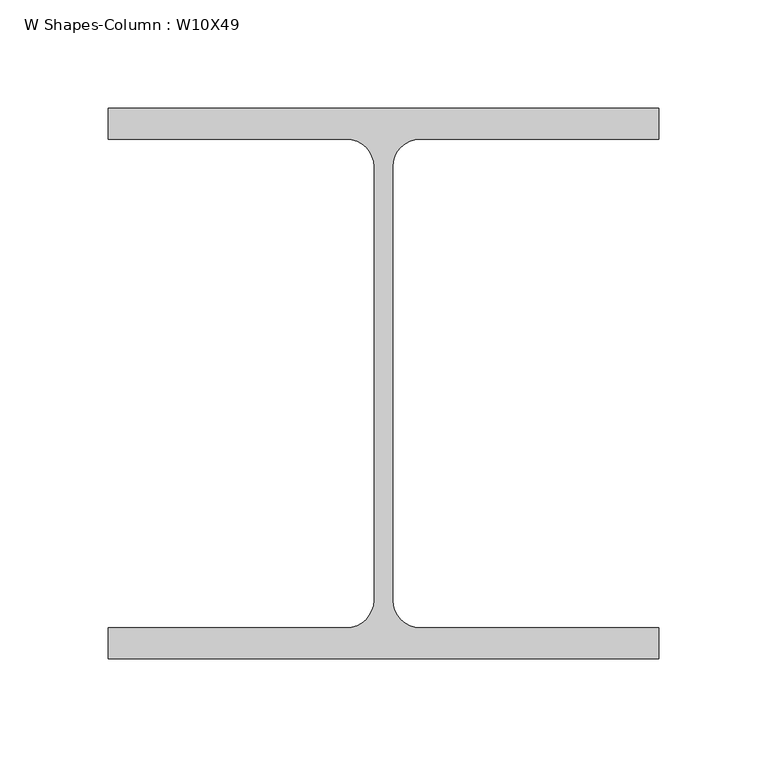
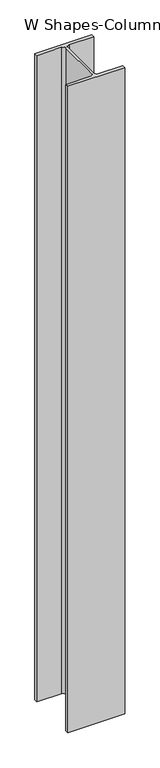
"""IFC4 building model written with IfcOpenShell, lengths in millimetres: column geometry, W Shapes-Column : W10X49."""

from ifc_helpers import new_model, si_unit, point, frame_2d, origin, origin_with_axes, place, context, project, spatial, polyline, circle_curve, trimmed, segment, composite_curve, outline, extrude, source, transform, mapped, element, save


def w_shapes_column_w10x49_a631470e(model_context):
    return source(origin(), model_context, "Body", "SweptSolid", [
        extrude(outline(composite_curve([segment(polyline([(127.0, 127.0), (127.0, 112.776), (17.018, 112.776)]), True, "CONTINUOUS"), segment(trimmed(circle_curve(frame_2d((17.018, 100.076)), 12.7), [point((17.018, 112.776))], [point((4.318, 100.076))], True, "CARTESIAN"), True, "CONTINUOUS"), segment(polyline([(4.318, 100.076), (4.318, -100.076)]), True, "CONTINUOUS"), segment(trimmed(circle_curve(frame_2d((17.018, -100.076)), 12.7), [point((4.318, -100.076))], [point((17.018, -112.776))], True, "CARTESIAN"), True, "CONTINUOUS"), segment(polyline([(17.018, -112.776), (127.0, -112.776), (127.0, -127.0), (-127.0, -127.0), (-127.0, -112.776), (-17.018, -112.776)]), True, "CONTINUOUS"), segment(trimmed(circle_curve(frame_2d((-17.018, -100.076)), 12.7), [point((-17.018, -112.776))], [point((-4.318, -100.076))], True, "CARTESIAN"), True, "CONTINUOUS"), segment(polyline([(-4.318, -100.076), (-4.318, 100.076)]), True, "CONTINUOUS"), segment(trimmed(circle_curve(frame_2d((-17.018, 100.076)), 12.7), [point((-4.318, 100.076))], [point((-17.018, 112.776))], True, "CARTESIAN"), True, "CONTINUOUS"), segment(polyline([(-17.018, 112.776), (-127.0, 112.776), (-127.0, 127.0), (127.0, 127.0)]), True, "CONTINUOUS")], self_intersect=False)), origin_with_axes(), (0.0, 0.0, 1.0), 3048.0),
    ])


if __name__ == "__main__":
    model = new_model("IFC4")
    model_context = context("Model", 3, world=origin())
    ifc_project = project(units=[si_unit("LENGTHUNIT", "METRE", prefix="MILLI")], contexts=[model_context])
    site = spatial("IfcSite", under=ifc_project)
    building = spatial("IfcBuilding", under=site)
    placement = place(None, origin())
    w_shapes_column_w10x49_shape = w_shapes_column_w10x49_a631470e(model_context)
    element("IfcColumn", 1, ObjectType="W Shapes-Column : W10X49", at=placement, inside=building, context=model_context, shape_type="MappedRepresentation", body=[
        mapped(w_shapes_column_w10x49_shape, transform((0.0, 0.0, 0.0), x_axis=(1.0, 0.0, 0.0), y_axis=(0.0, 1.0, 0.0), z_axis=(0.0, 0.0, 1.0))),
    ])
    save(model, "model.ifc")

# Revit data of these elements
# Type "W Shapes-Column : W10X49"
#   Section Name Key = "W10x49"
#   Assembly Code = "B10"
#   Width = 10.000"
#   Web Thickness = 0.340"
#   Web Fillet = 0.500"
#   Warping Constant = 2070.00 in⁶
#   Torsional Moment of Inertia = 1.39 in⁴
#   Section Area = 14.40 in²
#   Plastic Modulus weak axis = 28.30 in³
#   Plastic Modulus strong axis = 60.40 in³
#   Perimeter = 58.50 ft²/ft
#   Nominal Weight = 49.00 lbf/ft
#   Moment of Inertia weak axis = 93.40 in⁴
#   Moment of Inertia strong axis = 272.00 in⁴
#   Height = 10.000"
#   Flange Thickness = 0.560"
#   Elastic Modulus weak axis = 18.70 in³
#   Elastic Modulus strong axis = 54.60 in³
#   Centroid Vertical = 5.000"
#   Centroid Horizontal = 5.000"
#   Bolt Spacing = 0' - 5 1/2"
#   Structural Material [instance default] = Steel ASTM A992
#   Principal Axes Angle = 0
# Element 1 (IfcColumn, "W Shapes-Column : W10X49")
#   Materials on its faces: "Steel ASTM A992"
# Materials
#   "Steel ASTM A992": class "Metal", colour RGB 199 199 199, transparency 0, Description = "Structural steel 50ksi", Cost = 0
